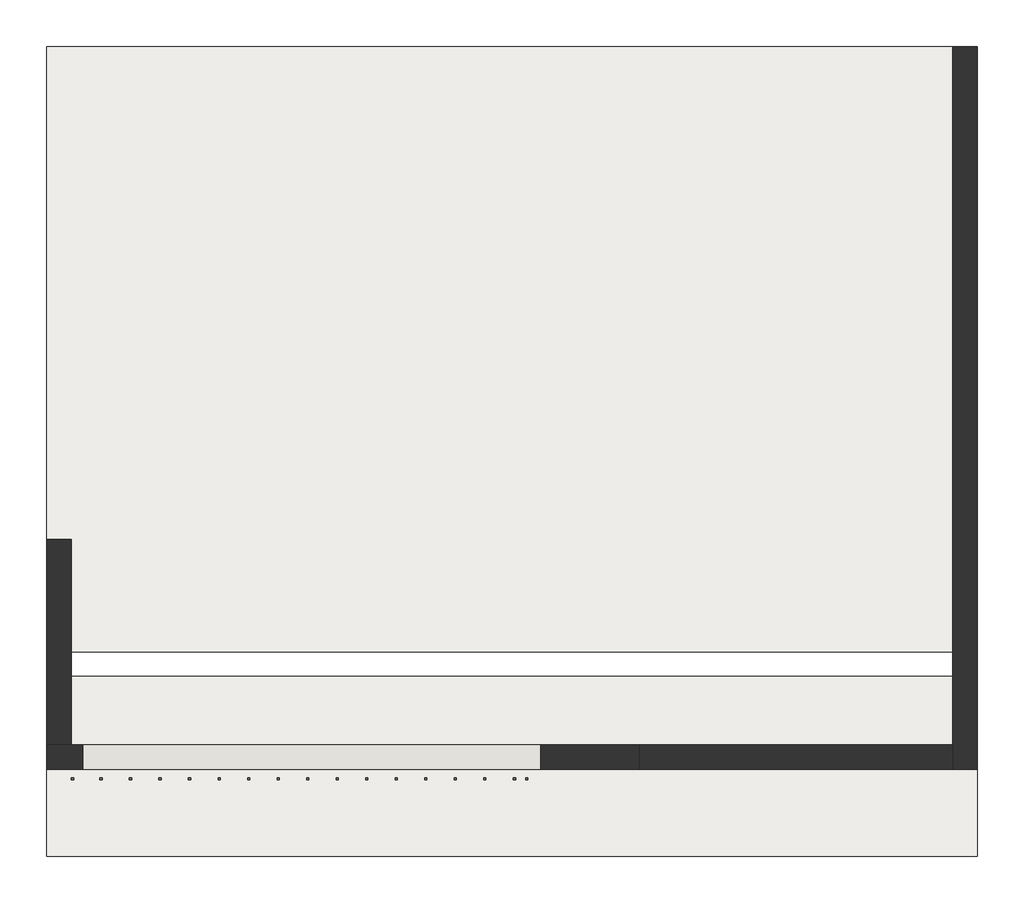
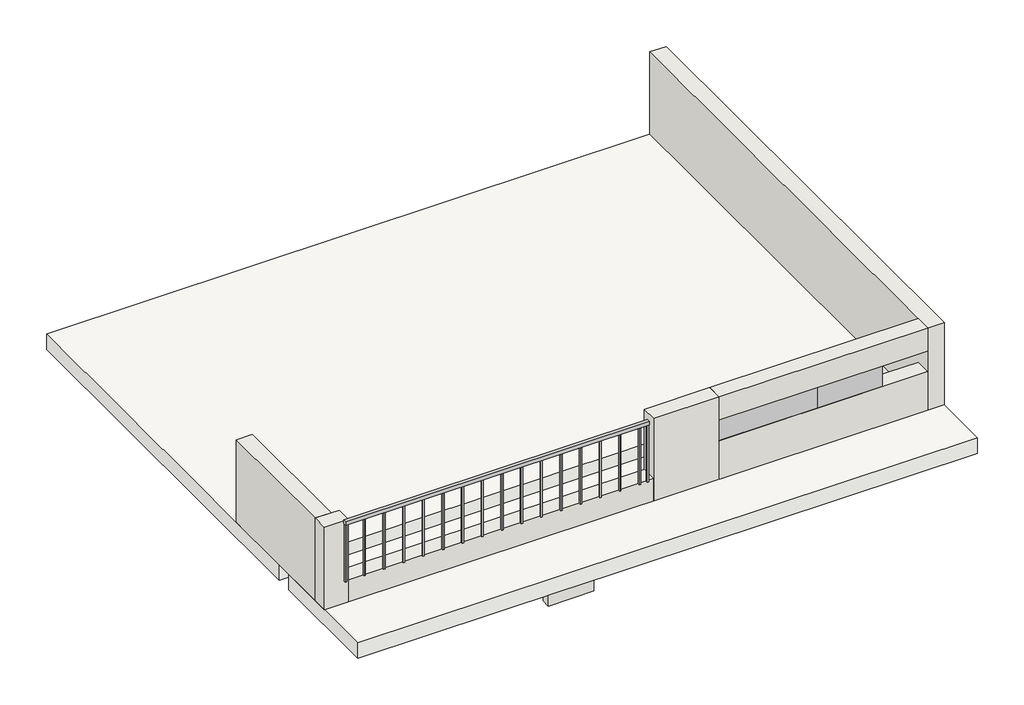
# One storey: 8 walls, 2 plates, 2 slabs, 1 railing.
"""IFC4 building model written with IfcOpenShell, lengths in millimetres."""

from ifc_helpers import new_model, si_unit, frame, origin, place, context, project, spatial, polyline, outline, extrude, faceted_brep, transform, mapped, element, save
from components import system_panel_glazed_57209e1b, system_panel_glazed_2e822fb3

model = new_model("IFC4")

# Units and contexts
model_context = context("Model", 3, world=origin())
ifc_project = project(units=[si_unit("LENGTHUNIT", "METRE", prefix="MILLI")], contexts=[model_context])

# Site, building, storey
site = spatial("IfcSite", under=ifc_project)
building = spatial("IfcBuilding", under=site)
storey = spatial("IfcBuildingStorey", under=building, Elevation=11887.2)

# Plates
placement = place(None, origin())
system_panel_glazed_shape = system_panel_glazed_57209e1b(model_context)
element("IfcPlate", 1, ObjectType="System Panel : Glazed", at=placement, inside=storey, context=model_context, shape_type="MappedRepresentation", body=[
    mapped(system_panel_glazed_shape, transform((6988.1055047, -7815.0053244, 12458.7752496), x_axis=(1.0, 0.0, 0.0), y_axis=(0.0, 1.0, 0.0), z_axis=(0.0, 0.0, 1.0))),
])
system_panel_glazed_2_shape = system_panel_glazed_2e822fb3(model_context)
element("IfcPlate", 2, ObjectType="System Panel : Glazed", at=placement, inside=storey, context=model_context, shape_type="MappedRepresentation", body=[
    mapped(system_panel_glazed_2_shape, transform((8132.6942325, -7815.0053244, 12458.7752496), x_axis=(1.0, 0.0, 0.0), y_axis=(0.0, 1.0, 0.0), z_axis=(0.0, 0.0, 1.0))),
])

# Railing
element("IfcRailing", 3, ObjectType="900mm", at=placement, inside=storey, context=model_context, shape_type="SweptSolid", body=[
    extrude(outline(polyline([(1011.7566492, -7906.2053244), (1011.7566492, -7856.2053244), (5259.9066492, -7856.2053244), (5259.9066492, -7906.2053244), (1011.7566492, -7906.2053244)])), frame((0.0, 0.0, 13124.3580822), z_axis=(0.0, 0.0, 1.0), x_axis=(1.0, 0.0, 0.0)), (0.0, 0.0, 1.0), 50.0),
    extrude(outline(polyline([(5126.7566492, -7871.2053244), (5146.7566492, -7871.2053244), (5146.7566492, -7891.2053244), (5126.7566492, -7891.2053244), (5126.7566492, -7871.2053244)])), frame((0.0, 0.0, 12274.3580822), z_axis=(0.0, 0.0, 1.0), x_axis=(1.0, 0.0, 0.0)), (0.0, 0.0, 1.0), 850.0),
    extrude(outline(polyline([(4851.7566492, -7871.2053244), (4871.7566492, -7871.2053244), (4871.7566492, -7891.2053244), (4851.7566492, -7891.2053244), (4851.7566492, -7871.2053244)])), frame((0.0, 0.0, 12274.3580822), z_axis=(0.0, 0.0, 1.0), x_axis=(1.0, 0.0, 0.0)), (0.0, 0.0, 1.0), 850.0),
    extrude(outline(polyline([(4576.7566492, -7871.2053244), (4596.7566492, -7871.2053244), (4596.7566492, -7891.2053244), (4576.7566492, -7891.2053244), (4576.7566492, -7871.2053244)])), frame((0.0, 0.0, 12274.3580822), z_axis=(0.0, 0.0, 1.0), x_axis=(1.0, 0.0, 0.0)), (0.0, 0.0, 1.0), 850.0),
    extrude(outline(polyline([(4301.7566492, -7871.2053244), (4321.7566492, -7871.2053244), (4321.7566492, -7891.2053244), (4301.7566492, -7891.2053244), (4301.7566492, -7871.2053244)])), frame((0.0, 0.0, 12274.3580822), z_axis=(0.0, 0.0, 1.0), x_axis=(1.0, 0.0, 0.0)), (0.0, 0.0, 1.0), 850.0),
    extrude(outline(polyline([(4026.7566492, -7871.2053244), (4046.7566492, -7871.2053244), (4046.7566492, -7891.2053244), (4026.7566492, -7891.2053244), (4026.7566492, -7871.2053244)])), frame((0.0, 0.0, 12274.3580822), z_axis=(0.0, 0.0, 1.0), x_axis=(1.0, 0.0, 0.0)), (0.0, 0.0, 1.0), 850.0),
    extrude(outline(polyline([(3751.7566492, -7871.2053244), (3771.7566492, -7871.2053244), (3771.7566492, -7891.2053244), (3751.7566492, -7891.2053244), (3751.7566492, -7871.2053244)])), frame((0.0, 0.0, 12274.3580822), z_axis=(0.0, 0.0, 1.0), x_axis=(1.0, 0.0, 0.0)), (0.0, 0.0, 1.0), 850.0),
    extrude(outline(polyline([(3476.7566492, -7871.2053244), (3496.7566492, -7871.2053244), (3496.7566492, -7891.2053244), (3476.7566492, -7891.2053244), (3476.7566492, -7871.2053244)])), frame((0.0, 0.0, 12274.3580822), z_axis=(0.0, 0.0, 1.0), x_axis=(1.0, 0.0, 0.0)), (0.0, 0.0, 1.0), 850.0),
    extrude(outline(polyline([(3201.7566492, -7871.2053244), (3221.7566492, -7871.2053244), (3221.7566492, -7891.2053244), (3201.7566492, -7891.2053244), (3201.7566492, -7871.2053244)])), frame((0.0, 0.0, 12274.3580822), z_axis=(0.0, 0.0, 1.0), x_axis=(1.0, 0.0, 0.0)), (0.0, 0.0, 1.0), 850.0),
    extrude(outline(polyline([(2926.7566492, -7871.2053244), (2946.7566492, -7871.2053244), (2946.7566492, -7891.2053244), (2926.7566492, -7891.2053244), (2926.7566492, -7871.2053244)])), frame((0.0, 0.0, 12274.3580822), z_axis=(0.0, 0.0, 1.0), x_axis=(1.0, 0.0, 0.0)), (0.0, 0.0, 1.0), 850.0),
    extrude(outline(polyline([(2651.7566492, -7871.2053244), (2671.7566492, -7871.2053244), (2671.7566492, -7891.2053244), (2651.7566492, -7891.2053244), (2651.7566492, -7871.2053244)])), frame((0.0, 0.0, 12274.3580822), z_axis=(0.0, 0.0, 1.0), x_axis=(1.0, 0.0, 0.0)), (0.0, 0.0, 1.0), 850.0),
    extrude(outline(polyline([(2376.7566492, -7871.2053244), (2396.7566492, -7871.2053244), (2396.7566492, -7891.2053244), (2376.7566492, -7891.2053244), (2376.7566492, -7871.2053244)])), frame((0.0, 0.0, 12274.3580822), z_axis=(0.0, 0.0, 1.0), x_axis=(1.0, 0.0, 0.0)), (0.0, 0.0, 1.0), 850.0),
    extrude(outline(polyline([(2101.7566492, -7871.2053244), (2121.7566492, -7871.2053244), (2121.7566492, -7891.2053244), (2101.7566492, -7891.2053244), (2101.7566492, -7871.2053244)])), frame((0.0, 0.0, 12274.3580822), z_axis=(0.0, 0.0, 1.0), x_axis=(1.0, 0.0, 0.0)), (0.0, 0.0, 1.0), 850.0),
    extrude(outline(polyline([(1826.7566492, -7871.2053244), (1846.7566492, -7871.2053244), (1846.7566492, -7891.2053244), (1826.7566492, -7891.2053244), (1826.7566492, -7871.2053244)])), frame((0.0, 0.0, 12274.3580822), z_axis=(0.0, 0.0, 1.0), x_axis=(1.0, 0.0, 0.0)), (0.0, 0.0, 1.0), 850.0),
    extrude(outline(polyline([(1551.7566492, -7871.2053244), (1571.7566492, -7871.2053244), (1571.7566492, -7891.2053244), (1551.7566492, -7891.2053244), (1551.7566492, -7871.2053244)])), frame((0.0, 0.0, 12274.3580822), z_axis=(0.0, 0.0, 1.0), x_axis=(1.0, 0.0, 0.0)), (0.0, 0.0, 1.0), 850.0),
    extrude(outline(polyline([(1276.7566492, -7871.2053244), (1296.7566492, -7871.2053244), (1296.7566492, -7891.2053244), (1276.7566492, -7891.2053244), (1276.7566492, -7871.2053244)])), frame((0.0, 0.0, 12274.3580822), z_axis=(0.0, 0.0, 1.0), x_axis=(1.0, 0.0, 0.0)), (0.0, 0.0, 1.0), 850.0),
    extrude(outline(polyline([(5239.9066492, -7871.2053244), (5259.9066492, -7871.2053244), (5259.9066492, -7891.2053244), (5239.9066492, -7891.2053244), (5239.9066492, -7871.2053244)])), frame((0.0, 0.0, 12274.3580822), z_axis=(0.0, 0.0, 1.0), x_axis=(1.0, 0.0, 0.0)), (0.0, 0.0, 1.0), 850.0),
    extrude(outline(polyline([(1011.7566492, -7871.2053244), (1031.7566492, -7871.2053244), (1031.7566492, -7891.2053244), (1011.7566492, -7891.2053244), (1011.7566492, -7871.2053244)])), frame((0.0, 0.0, 12274.3580822), z_axis=(0.0, 0.0, 1.0), x_axis=(1.0, 0.0, 0.0)), (0.0, 0.0, 1.0), 850.0),
])

# Slabs
element("IfcSlab", 4, ObjectType="9\"", at=placement, inside=storey, context=model_context, shape_type="Brep", body=[
    faceted_brep([(9448.1305046, -6926.0053244, 11658.6), (9448.1305046, -8602.4053244, 11658.6), (780.1132171, -8602.4053244, 11658.6), (780.1132171, -6926.0053244, 11658.6), (9448.1305046, -6926.0053244, 11887.2), (788.1495839, -6926.0053244, 11887.2), (780.1132171, -6926.0053244, 11887.2), (780.1132171, -8602.4053244, 11887.2), (9448.1305046, -8602.4053244, 11887.2), (9448.1305046, -7793.6953528, 11887.2)], [[[0, 1, 2, 3]], [[4, 5, 6, 7, 8, 9]], [[1, 0, 4, 9, 8]], [[2, 1, 8, 7]], [[3, 2, 7, 6]], [[0, 3, 6, 5, 4]]]),
])
element("IfcSlab", 5, ObjectType="9\"", at=placement, inside=storey, context=model_context, shape_type="Brep", body=[
    faceted_brep([(9448.1305046, -1058.6053244, 11658.6), (9448.1305046, -1515.8053244, 11658.6), (9448.1305046, -6697.4053244, 11658.6), (9219.5305046, -6697.4053244, 11658.6), (780.1132171, -6697.4053244, 11658.6), (780.1132171, -1058.6053244, 11658.6), (9448.1305046, -1058.6053244, 11887.2), (9219.5305046, -1058.6053244, 11887.2), (780.1132171, -1058.6053244, 11887.2), (780.1132171, -6697.4053244, 11887.2), (9448.1305046, -6697.4053244, 11887.2)], [[[0, 1, 2, 3, 4, 5]], [[6, 7, 8, 9, 10]], [[2, 1, 0, 6, 10]], [[4, 3, 2, 10, 9]], [[5, 4, 9, 8]], [[0, 5, 8, 7, 6]]]),
])

# Walls
element("IfcWall", 6, ObjectType="5\"", at=placement, inside=storey, context=model_context, shape_type="SweptSolid", body=[
    extrude(outline(polyline([(4080.8441177, -8602.4053244), (3443.6004948, -8602.4053244), (3443.6004948, -8475.4053244), (4080.8441177, -8475.4053244), (4080.8441177, -8602.4053244)])), frame((0.0, 0.0, 11500.8069379), z_axis=(0.0, 0.0, 1.0), x_axis=(1.0, 0.0, 0.0)), (0.0, 0.0, 1.0), 157.7930621),
])
element("IfcWall", 7, ObjectType="9\"", at=placement, inside=storey, context=model_context, shape_type="Brep", body=[
    faceted_brep([(5384.1305046, -7793.6953528, 11887.2), (6298.5305046, -7793.6953528, 11887.2), (6298.5305046, -7793.6953528, 12458.7752496), (6298.5305046, -7793.6953528, 12763.5752496), (6298.5305046, -7793.6953528, 13106.4), (5384.1305046, -7793.6953528, 13106.4), (5384.1305046, -7793.6953528, 12217.4), (5384.1305046, -7565.0953528, 11887.2), (5384.1305046, -7565.0953528, 12217.4), (5384.1305046, -7565.0953528, 13106.4), (6298.5305046, -7565.0953528, 13106.4), (6298.5305046, -7565.0953528, 12763.5752496), (6298.5305046, -7565.0953528, 12458.7752496), (6298.5305046, -7565.0953528, 11887.2)], [[[0, 1, 2, 3, 4, 5, 6]], [[7, 8, 9, 10, 11, 12, 13]], [[1, 0, 7, 13]], [[4, 3, 2, 1, 13, 12, 11, 10]], [[5, 4, 10, 9]], [[0, 6, 5, 9, 8, 7]]]),
])
element("IfcWall", 8, ObjectType="9\"", at=placement, inside=storey, context=model_context, shape_type="SweptSolid", body=[
    extrude(outline(polyline([(5384.1305046, -7793.6953528), (1115.847284, -7793.6953528), (1115.847284, -7565.0953528), (5384.1305046, -7565.0953528), (5384.1305046, -7793.6953528)])), frame((0.0, 0.0, 11887.2), z_axis=(0.0, 0.0, 1.0), x_axis=(1.0, 0.0, 0.0)), (0.0, 0.0, 1.0), 330.2),
])
element("IfcWall", 9, ObjectType="9\"", at=placement, inside=storey, context=model_context, shape_type="Brep", body=[
    faceted_brep([(780.1132171, -7793.6953528, 11887.2), (1115.847284, -7793.6953528, 11887.2), (1115.847284, -7793.6953528, 12217.4), (1115.847284, -7793.6953528, 13106.4), (780.1132171, -7793.6953528, 13106.4), (780.1132171, -7565.0953528, 11887.2), (780.1132171, -7565.0953528, 13106.4), (1008.7132171, -7565.0953528, 13106.4), (1115.847284, -7565.0953528, 13106.4), (1115.847284, -7565.0953528, 12217.4), (1115.847284, -7565.0953528, 11887.2), (1008.7132171, -7565.0953528, 11887.2)], [[[0, 1, 2, 3, 4]], [[5, 6, 7, 8, 9, 10, 11]], [[1, 0, 5, 11, 10]], [[3, 2, 1, 10, 9, 8]], [[4, 3, 8, 7, 6]], [[0, 4, 6, 5]]]),
])
element("IfcWall", 10, ObjectType="9\"", at=placement, inside=storey, context=model_context, shape_type="SweptSolid", body=[
    extrude(outline(polyline([(1008.7132171, -5652.7354899), (1008.7132171, -7565.0953528), (780.1132171, -7565.0953528), (780.1132171, -5652.7354899), (1008.7132171, -5652.7354899)])), frame((0.0, 0.0, 11887.2), z_axis=(0.0, 0.0, 1.0), x_axis=(1.0, 0.0, 0.0)), (0.0, 0.0, 1.0), 1219.2),
])
element("IfcWall", 11, ObjectType="9\"", at=placement, inside=storey, context=model_context, shape_type="Brep", body=[
    faceted_brep([(9448.1305046, -7793.6953528, 11887.2), (9448.1305046, -6926.0053244, 11887.2), (9448.1305046, -6697.4053244, 11887.2), (9448.1305046, -1058.6053244, 11887.2), (9448.1305046, -1058.6053244, 13106.4), (9448.1305046, -7793.6953528, 13106.4), (9219.5305046, -7793.6953528, 11887.2), (9219.5305046, -7793.6953528, 12458.7752496), (9219.5305046, -7793.6953528, 12763.5752496), (9219.5305046, -7793.6953528, 13106.4), (9219.5305046, -7565.0953528, 13106.4), (9219.5305046, -1058.6053244, 13106.4), (9219.5305046, -1058.6053244, 11887.2), (9219.5305046, -7565.0953528, 11887.2)], [[[0, 1, 2, 3, 4, 5]], [[6, 7, 8, 9, 10, 11, 12, 13]], [[3, 2, 1, 0, 6, 13, 12]], [[4, 3, 12, 11]], [[5, 4, 11, 10, 9]], [[0, 5, 9, 8, 7, 6]]]),
])
element("IfcWall", 12, ObjectType="9\"", at=placement, inside=storey, context=model_context, shape_type="Brep", body=[
    faceted_brep([(6298.5305046, -7793.6953528, 11887.2), (9219.5305046, -7793.6953528, 11887.2), (9219.5305046, -7793.6953528, 12458.7752496), (8587.7079602, -7793.6953528, 12458.7752496), (6298.5305046, -7793.6953528, 12458.7752496), (6298.5305046, -7565.0953528, 11887.2), (6298.5305046, -7565.0953528, 12458.7752496), (8587.7079602, -7565.0953528, 12458.7752496), (9219.5305046, -7565.0953528, 12458.7752496), (9219.5305046, -7565.0953528, 11887.2)], [[[0, 1, 2, 3, 4]], [[5, 6, 7, 8, 9]], [[1, 0, 5, 9]], [[2, 1, 9, 8]], [[4, 3, 2, 8, 7, 6]], [[0, 4, 6, 5]]]),
])
element("IfcWall", 13, ObjectType="9\"", at=placement, inside=storey, context=model_context, shape_type="Brep", body=[
    faceted_brep([(6298.5305046, -7793.6953528, 12763.5752496), (8587.7079602, -7793.6953528, 12763.5752496), (9219.5305046, -7793.6953528, 12763.5752496), (9219.5305046, -7793.6953528, 13106.4), (6298.5305046, -7793.6953528, 13106.4), (6298.5305046, -7565.0953528, 12763.5752496), (6298.5305046, -7565.0953528, 13106.4), (9219.5305046, -7565.0953528, 13106.4), (9219.5305046, -7565.0953528, 12763.5752496), (8587.7079602, -7565.0953528, 12763.5752496)], [[[0, 1, 2, 3, 4]], [[5, 6, 7, 8, 9]], [[2, 1, 0, 5, 9, 8]], [[4, 3, 7, 6]], [[0, 4, 6, 5]], [[3, 2, 8, 7]]]),
])

save(model, "model.ifc")

# Revit data of these elements
# Type "System Panel : Glazed"
#   Keynote = "H11"
#   Construction Type Id = "GSP4R"
#   Analytic Construction = "1/8 in Pilkington single glazing"
#   Visual Light Transmittance = 0.9
#   Solar Heat Gain Coefficient = 0.86
#   Heat Transfer Coefficient (U) = 6.7069 W/(m²·K)
#   Define Thermal Properties by = 1
# Type "900mm"
#   built-in parameter 1008612 = 0.019685 (stored number, unit not read)
#   built-in parameter 1008611 = 0.019685 (stored number, unit not read)
#   built-in parameter 1008609 = 0.902231 (stored number, unit not read)
#   built-in parameter 1008604 = 0.19685 (stored number, unit not read)
#   built-in parameter 1008603 = 0.164042 (stored number, unit not read)
#   Railing Height = 2' - 11.43307"
#   built-in parameter 1008630 = 2
#   built-in parameter 1008610 = 2
#   built-in parameter 1008608 = 1
#   built-in parameter 1008618 = Baluster_Square : 20mm
# Type "9\""
#   Keynote = "E60/130"
#   Function = 0
#   Layers, outside or top first: 0' - 9" "Concrete, Precast" (function 1)
# Type "5\""
#   Keynote = "F10"
#   Layers, outside or top first: 0' - 5" "Concrete" (function 1)
# Type "9\""
#   Keynote = "F10"
#   Layers, outside or top first: 0' - 9" "Concrete" (function 1)
# Elements 1, 2 (IfcPlate, "System Panel : Glazed")
#   Phase Created = New Construction
#   Materials on its faces: "Glass"
# Element 3 (IfcRailing, "900mm")
#   built-in parameter 1008621 = 1.2702 (stored number, unit not read)
#   Phase Created = New Construction
# Element 4 (IfcSlab, "9\"")
#   Height Offset From Level = 0' - 0"
#   Phase Created = New Construction
#   Materials on its faces: "Concrete, Precast", "Earth", "Gypsum Wall Board"
# Element 5 (IfcSlab, "9\"")
#   Height Offset From Level = 0' - 0"
#   Phase Created = New Construction
#   Materials on its faces: "Concrete, Precast", "Gypsum Wall Board"
# Element 6 (IfcWall, "5\"")
#   built-in parameter 1001111 = -1' - 3.21233"
#   Top Offset = -12' - 6"
#   Base Offset = -1' - 3.21233"
#   wall height = 0' - 6.21233"
#   Phase Created = New Construction
#   Base Constraint = ROOF LEV
#   Materials on its faces: "Concrete"
# Elements 7, 10 (IfcWall, "9\"")
#   Top Offset = 0' - 0"
#   Base Offset = 0' - 0"
#   wall height = 4' - 0"
#   Phase Created = New Construction
#   Base Constraint = ROOF LEV
#   Materials on its faces: "Concrete", "Earth"
# Element 8 (IfcWall, "9\"")
#   Top Offset = 0' - 0"
#   Base Offset = 0' - 0"
#   Unconnected Height = 1' - 1"
#   wall height = 1' - 1"
#   Phase Created = New Construction
#   Base Constraint = ROOF LEV
#   Materials on its faces: "Concrete"
# Element 9 (IfcWall, "9\"")
#   Top Offset = 0' - 0"
#   Base Offset = 0' - 0"
#   wall height = 4' - 0"
#   Phase Created = New Construction
#   Base Constraint = ROOF LEV
#   Materials on its faces: "Earth", "Concrete"
# Element 11 (IfcWall, "9\"")
#   Top Offset = 0' - 0"
#   Base Offset = 0' - 0"
#   wall height = 4' - 0"
#   Phase Created = New Construction
#   Base Constraint = ROOF LEV
#   Materials on its faces: "Concrete", "Gypsum Wall Board", "Earth"
# Element 12 (IfcWall, "9\"")
#   Top Offset = -2' - 1.49704"
#   Base Offset = 0' - 0"
#   wall height = 1' - 10.50296"
#   Phase Created = New Construction
#   Base Constraint = ROOF LEV
#   Materials on its faces: "Concrete", "Earth"
# Element 13 (IfcWall, "9\"")
#   built-in parameter 1001111 = 2' - 10.50296"
#   Top Offset = -7' - 9"
#   Base Offset = 2' - 10.50296"
#   wall height = 1' - 1.49704"
#   Phase Created = New Construction
#   Base Constraint = ROOF LEV
#   Materials on its faces: "Concrete", "Earth"
# Materials
#   "Concrete, Precast": class "Concrete", colour RGB 192 192 192, transparency 0, Description = "Precast concrete", Cost = 0
#   "Concrete": class "Concrete", colour RGB 120 120 120, transparency 0, Description = "Portland Cement Concrete", Cost = 0
#   "Glass": class "Glass", colour RGB 0 128 192, transparency 0.9, Description = "Soda Lime Glass", Cost = 0
#   "Earth": class "Generic", colour RGB 97 75 62, transparency 0, Description = "Soil", Cost = 0
#   "Gypsum Wall Board": class "Generic", colour RGB 249 249 249, transparency 0, Description = "Gypsum Wall Board", Cost = 0
